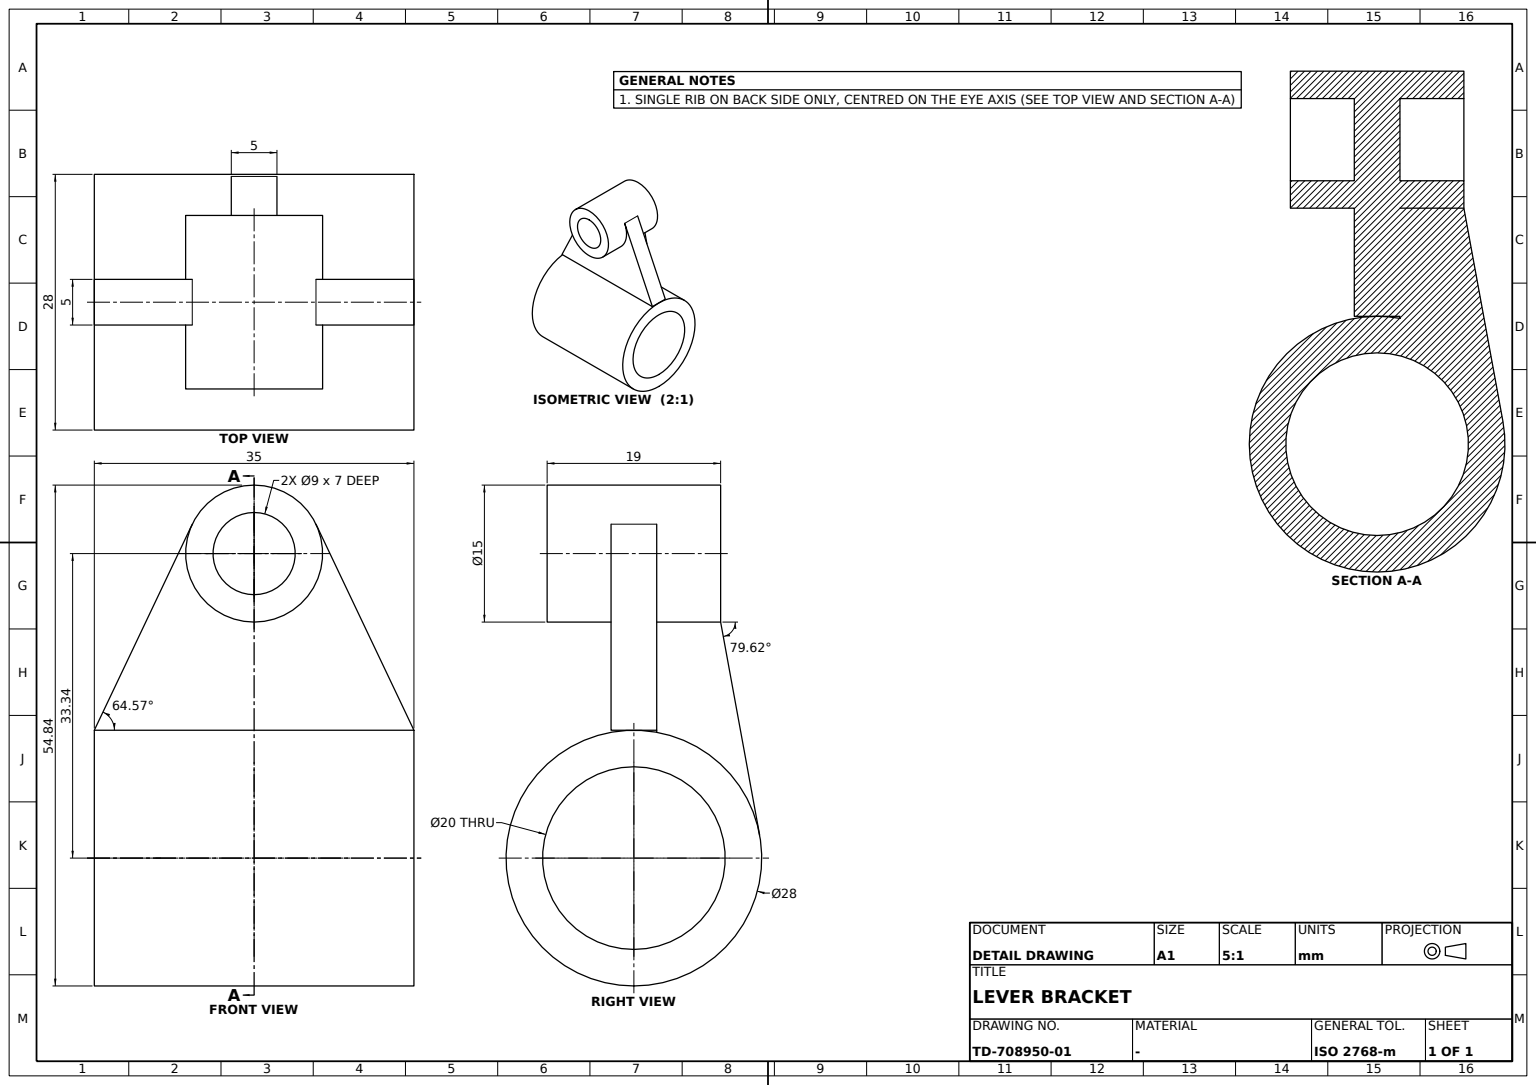
CATIA V5 part; units mm, degrees
sketch "Sketch1" plane through (0, 0, 0) normal (1, 0, 0) x (0, 1, 0)
  circle A0 centre (0, 0) radius 14
  circle A1 centre (0, 0) radius 10
  dimension "radius A1" = 10
  dimension "radius A0" = 14
extrude "Pad1" add sketch "Sketch1" along normal mid plane 35
sketch "Sketch2" plane through (0, 0, 0) normal (0, 1, 0) x (-1, 0, 0)
  circle A0 centre (0, 33.342) radius 7.5
  point P0 (0, 33.342)
  circle A1 centre (0, 33.342) radius 4.5
  dimension "radius A1" = 4.5
  dimension "radius A0" = 7.5
  constraint coincidence P0 y-axis
extrude "Pad2" add sketch "Sketch2" along normal mid plane 19
sketch "Sketch3" plane through (0, 0, 0) normal (0, 1, 0) x (-1, 0, 0)
  line L0 (-6.7735, 36.5623) -> (-17.5, 14)
  line L1 (-17.5, 14) -> (17.5, 14)
  line L2 (17.5, 14) -> (6.7735, 36.5623)
  circle A0 centre (0, 33.342) radius 7.5 construction
  arc A1 (6.7735, 36.5623) -> (-6.7735, 36.5623) centre (0, 33.342) ccw
  point P0 (6.7735, 36.5623)
  point P1 (-6.7735, 36.5623)
  constraint horizontal L1 x-axis
  constraint tangency A0 L0
  constraint tangency L2 A0
  constraint coincidence A0 P0
  constraint coincidence A0 P1
extrude "Pad3" add sketch "Sketch3" along normal mid plane 5
sketch "Sketch4" plane through (0, 0, 0) normal (1, 0, 0) x (0, 1, 0)
  line L0 (2.5, 25.842) -> (9.5, 25.842)
  line L1 (9.5, 25.842) -> (13.7709, 2.5221)
  line L2 (2.5, 25.842) -> (2.5, 13.775)
  point P0 (2.5, 13.775)
  line L3 (2.5, 36.5623) -> (2.5, 14) construction
  circle A0 centre (0, 0) radius 14 construction
  arc A1 (13.7709, 2.5221) -> (2.5, 13.775) centre (0, 0) ccw
  constraint vertical L2 y-axis
  constraint coincidence L3 L2
  constraint coincidence P0 A0
  constraint tangency L1 A0
extrude "Pad4" add sketch "Sketch4" along normal mid plane 5
